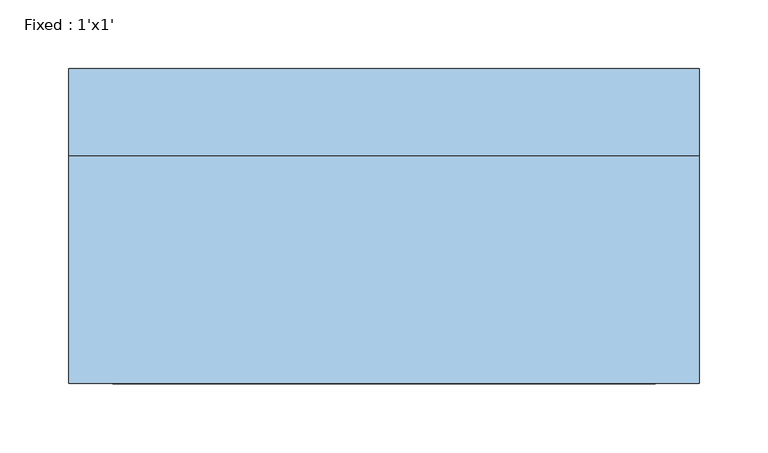
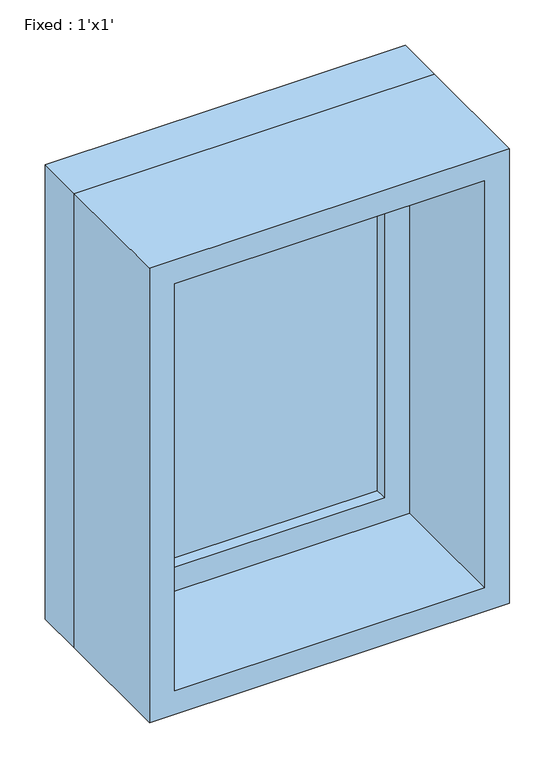
"""IFC4 building model written with IfcOpenShell, lengths in millimetres: window geometry, Fixed : 1'x1'."""

from ifc_helpers import new_model, si_unit, frame, origin, place, context, project, spatial, polyline, outline, extrude, source, transform, mapped, element, save


def fixed_1_x1_542de505(model_context):
    return source(origin(), model_context, "Body", "SweptSolid", [
        extrude(outline(polyline([(127.0, 66.675), (-203.2, 66.675), (-203.2, 79.375), (127.0, 79.375), (127.0, 66.675)])), frame((0.0, 0.0, 368.3), z_axis=(0.0, 0.0, 1.0), x_axis=(1.0, 0.0, 0.0)), (0.0, 0.0, 1.0), 482.6),
        extrude(outline(polyline([(895.35, -247.65), (323.85, -247.65), (323.85, 171.45), (895.35, 171.45), (895.35, -247.65)]), holes=[polyline([(850.9, -203.2), (850.9, 127.0), (368.3, 127.0), (368.3, -203.2), (850.9, -203.2)])]), frame((0.0, 50.8, 0.0), z_axis=(0.0, 1.0, 0.0), x_axis=(0.0, 0.0, 1.0)), (0.0, 0.0, 1.0), 44.45),
        extrude(outline(polyline([(914.4, -266.7), (304.8, -266.7), (304.8, 190.5), (914.4, 190.5), (914.4, -266.7)]), holes=[polyline([(882.65, -234.95), (882.65, 158.75), (336.55, 158.75), (336.55, -234.95), (882.65, -234.95)])]), frame((0.0, -114.3, 0.0), z_axis=(0.0, 1.0, 0.0), x_axis=(0.0, 0.0, 1.0)), (0.0, 0.0, 1.0), 165.1),
        extrude(outline(polyline([(914.4, 190.5), (914.4, -266.7), (304.8, -266.7), (304.8, 190.5), (914.4, 190.5)]), holes=[polyline([(895.35, 171.45), (323.85, 171.45), (323.85, -247.65), (895.35, -247.65), (895.35, 171.45)])]), frame((0.0, 50.8, 0.0), z_axis=(0.0, 1.0, 0.0), x_axis=(0.0, 0.0, 1.0)), (0.0, 0.0, 1.0), 63.5),
    ])


if __name__ == "__main__":
    model = new_model("IFC4")
    model_context = context("Model", 3, world=origin())
    ifc_project = project(units=[si_unit("LENGTHUNIT", "METRE", prefix="MILLI")], contexts=[model_context])
    site = spatial("IfcSite", under=ifc_project)
    building = spatial("IfcBuilding", under=site)
    placement = place(None, origin())
    fixed_1_x1_shape = fixed_1_x1_542de505(model_context)
    element("IfcWindow", 1, ObjectType="Fixed : 1'x1'", at=placement, inside=building, context=model_context, shape_type="MappedRepresentation", body=[
        mapped(fixed_1_x1_shape, transform((0.0, 0.0, 0.0), x_axis=(1.0, 0.0, 0.0), y_axis=(0.0, 1.0, 0.0), z_axis=(0.0, 0.0, 1.0))),
    ])
    save(model, "model.ifc")

# Revit data of these elements
# Type "Fixed : 1'x1'"
#   Type Mark = "18"
#   Construction Type Id = "GSP4R"
#   Assembly Code = "B2020100"
#   Analytic Construction = "1/8 in Pilkington single glazing"
#   Visual Light Transmittance = 0.9
#   Solar Heat Gain Coefficient = 0.78
#   Heat Transfer Coefficient (U) = 0.6496 BTU/(h·ft²·°F)
#   Height = 2' - 0"
#   Default Sill Height = 1' - 0"
#   Width = 1' - 6"
#   Window Inset = 0' - 0 3/4"
#   Define Thermal Properties by = 1
#   Glass Pane Material = Glass
#   Sash Material = door black
#   Wall Closure = (empty or 0)
# Element 1 (IfcWindow, "Fixed : 1'x1'")
#   Materials on its faces: "door black", "Glass"
# Materials
#   "Glass": class "Glass", colour RGB 0 128 192, transparency 0.75, Description = "Soda Lime Glass", Cost = 0
#   "door black": class "Generic", colour RGB 120 120 120, transparency 0, Cost = 0
